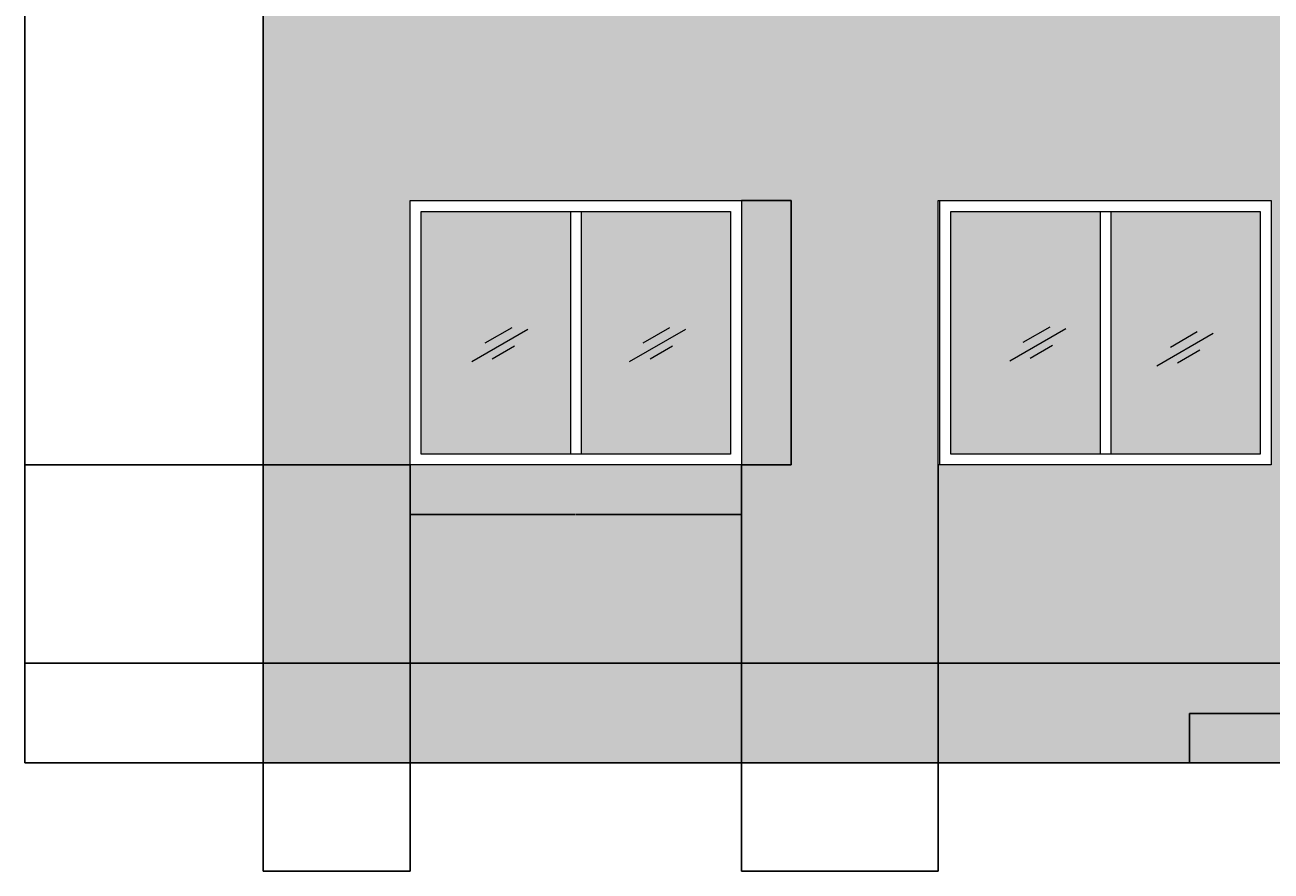
# Model space of a CAD drawing. Units: millimetres. Extents: x 2511 to 24632, y 2213 to 12972.
# Tile 4 of 5: x 13664 to 19414, y 2507 to 6412. Entities that reach past the tile are written whole.
import ezdxf

# ---------------------------------------------------------------- set-up
doc = ezdxf.new("R2010")
doc.units = ezdxf.units.MM
for name, color, linetype, lineweight in [('A-ANNO-DIMS', 2, 'Continuous', 18), ('A-BASE-PATT', 9, 'Continuous', 9), ('A-ELEV', 7, 'Continuous', 25), ('A-ELEV-GLAZ', 7, 'Continuous', 18), ('A-ELEV-PATT', 13, 'Continuous', 9)]:
    doc.layers.add(name, color=color, linetype=linetype, lineweight=lineweight)
doc.layers.add('A-GLAZ-PATT', color=141, linetype='Continuous', lineweight=9, true_color=0xadddf7)
doc.styles.get("Standard").update_dxf_attribs({"font": 'arial.ttf'})
doc.dimstyles.get("Standard").update_dxf_attribs({"dimtxt": 0.18, "dimasz": 0.18, "dimexe": 0.18, "dimexo": 0.0625, "dimgap": 0.09, "dimtad": 0, "dimtih": 1, "dimtoh": 1, "dimdec": 4, "dimzin": 0, "dimdsep": 46, "dimtxsty": 'Standard', "dimcen": 0.09, "dimadec": 0, "dimazin": 0, "dimtfac": 1, "dimtdec": 4, "dimtofl": 0, "dimtmove": 0, "dimatfit": 3, "dimfxl": 1, "dimtolj": 1, "dimtzin": 0, "dimarcsym": 0})

# ---------------------------------------------------------------- blocks, each defined once
blk = doc.blocks.new('WINDOW-FRAME-1528-ELEV')
for p, q in [((3.45580574503e-05, -0.0004698816292148), (3.45580574503e-05, 1219.999530118371)), ((3.45580574503e-05, 1219.999530118371), (1527.988197152912, 1219.999530118371)), ((1527.988197152912, 1219.999530118371), (1527.988197152912, -0.0004698816292148)), ((738.9941158554847, 1169.999530118371), (738.9941158554847, 49.99953011837078)), ((788.9941158554847, 1169.999530118371), (788.9941158554847, 49.99953011837078)), ((1527.988197152912, -0.0004698816292148), (3.45580574503e-05, -0.0004698816292148))]:
    blk.add_line(p, q)
for points in [[(3.45580574503e-05, 1219.999530118371), (1527.988197152912, 1219.999530118371), (1527.988197152912, -0.0004698816292148), (3.45580574503e-05, -0.0004698816292148)], [(50.00003455805745, 1169.999530118371), (1477.988197152912, 1169.999530118371), (1477.988197152912, 49.99953011837078), (50.00003455805745, 49.99953011837078)]]:
    blk.add_lwpolyline(points, close=True)
blk = doc.blocks.new('WINDOW-FRAME-1536-ELEV')
for p, q in [((-0.0001940248657775, -0.0004698816292148), (-0.0001940248657775, 1219.999530118371)), ((-0.0001940248657775, 1219.999530118371), (1536.172544795805, 1219.999530118371)), ((1536.172544795805, 1219.999530118371), (1536.172544795805, -0.0004698816292148)), ((747.1784634983741, 1169.999530118371), (747.1784634983741, 49.99953011837078)), ((797.1784634983742, 1169.999530118371), (797.1784634983742, 49.99953011837078)), ((1536.172544795805, -0.0004698816292148), (-0.0001940248657775, -0.0004698816292148))]:
    blk.add_line(p, q)
for points in [[(8.184382200950495, 1219.999530118371), (1536.172544795805, 1219.999530118371), (1536.172544795805, -0.0004698816292148), (8.184382200950495, -0.0004698816292148)], [(58.1843822009505, 1169.999530118371), (1486.172544795805, 1169.999530118371), (1486.172544795805, 49.99953011837078), (58.1843822009505, 49.99953011837078)]]:
    blk.add_lwpolyline(points, close=True)
blk = doc.blocks.new('GLASS-REFLECTION')
for p, q in [((0.000348498528183, -0.0002333358270334), (259.2110812861792, 149.655153015964)), ((62.47510116635385, 86.0291626371336), (186.2553756901197, 157.4937374537958)), ((94.69077173755068, 13.20916119840785), (197.7341820365163, 72.70130187273116))]:
    blk.add_line(p, q)
blk = doc.blocks.new('*D31')
at = {"layer": 'A-ANNO-DIMS', "color": 0, "lineweight": -2, "transparency": 16777216}
for p, q in [((15441.81503455806, 4381.154030118369), (15441.81503455806, 4151.838305729142)), ((16969.80319715291, 4381.154030118369), (16969.80319715291, 4151.838305729142)), ((15441.99503455805, 4152.018305729142), (16204.67128502329, 4152.018305729142)), ((16969.62319715291, 4152.018305729142), (16206.94694668768, 4152.018305729142))]:
    blk.add_line(p, q, dxfattribs=at)
at = {"layer": 'A-ANNO-DIMS', "color": 0, "transparency": 16777216}
for points in [[(15441.99503455805, 4152.048305729141), (15441.99503455805, 4151.988305729141), (15441.81503455806, 4152.018305729142)], [(16969.62319715291, 4152.048305729141), (16969.62319715291, 4151.988305729141), (16969.80319715291, 4152.018305729142)]]:
    blk.add_solid(points, dxfattribs=at)
at = {"layer": 'Defpoints', "color": 0, "transparency": 16777216}
for p in [(15441.81503455806, 4381.216530118369), (16969.80319715291, 4381.216530118369), (16969.80319715291, 4152.018305729142)]:
    blk.add_point(p, dxfattribs=at)
at = {"layer": 'A-ANNO-DIMS', "color": 0, "transparency": 16777216, "insert": (16205.80911585548, 4152.018305729142), "char_height": 0.18, "attachment_point": 5}
blk.add_mtext('\\A1;FRAME 1528 TYP.', dxfattribs=at)
blk = doc.blocks.new('*D32')
at = {"layer": 'A-ANNO-DIMS', "color": 0, "lineweight": -2, "transparency": 16777216}
for p, q in [((16969.86569715292, 5601.216530118371), (17199.18142154215, 5601.216530118371)), ((17199.00142154215, 5601.036530118371), (17199.00142154215, 4991.398433256161)), ((17199.00142154215, 4381.396530118371), (17199.00142154215, 4991.034626980582)), ((16969.86569715292, 4381.216530118371), (17199.18142154215, 4381.216530118371))]:
    blk.add_line(p, q, dxfattribs=at)
at = {"layer": 'A-ANNO-DIMS', "color": 0, "transparency": 16777216}
for points in [[(17198.97142154215, 5601.036530118371), (17199.03142154215, 5601.036530118371), (17199.00142154215, 5601.216530118371)], [(17198.97142154215, 4381.396530118371), (17199.03142154215, 4381.396530118371), (17199.00142154215, 4381.216530118371)]]:
    blk.add_solid(points, dxfattribs=at)
at = {"layer": 'Defpoints', "color": 0, "transparency": 16777216}
for p in [(16969.80319715292, 5601.216530118371), (17199.00142154215, 5601.216530118371), (16969.80319715292, 4381.216530118371)]:
    blk.add_point(p, dxfattribs=at)
at = {"layer": 'A-ANNO-DIMS', "color": 0, "transparency": 16777216, "insert": (17199.00142154215, 4991.216530118366), "char_height": 0.18, "attachment_point": 5}
blk.add_mtext('\\A1;1220 TYP.', dxfattribs=at)
blk = doc.blocks.new('*D66')
at = {"layer": 'A-ANNO-DIMS', "color": 0, "lineweight": -2, "transparency": 16777216}
for p, q in [((14762.747297, 3466.216530000002), (13663.87979700001, 3466.216530000002)), ((13664.05979700001, 3466.036530000002), (13664.05979700001, 3236.398433137792)), ((13664.05979700001, 3006.396530000001), (13664.05979700001, 3236.034626862212)), ((14762.747297, 3006.216530000001), (13663.87979700001, 3006.216530000001))]:
    blk.add_line(p, q, dxfattribs=at)
at = {"layer": 'A-ANNO-DIMS', "color": 0, "transparency": 16777216}
for points in [[(13664.02979700001, 3466.036530000002), (13664.08979700001, 3466.036530000002), (13664.05979700001, 3466.216530000002)], [(13664.02979700001, 3006.396530000001), (13664.08979700001, 3006.396530000001), (13664.05979700001, 3006.216530000001)]]:
    blk.add_solid(points, dxfattribs=at)
at = {"layer": 'Defpoints', "color": 0, "transparency": 16777216}
for p in [(13664.05979700001, 3466.216530000002), (14762.809797, 3466.216530000002), (14762.809797, 3006.216530000001)]:
    blk.add_point(p, dxfattribs=at)
at = {"layer": 'A-ANNO-DIMS', "color": 0, "transparency": 16777216, "insert": (13664.05979700001, 3236.216529999997), "char_height": 0.18, "attachment_point": 5}
blk.add_mtext('\\A1;460', dxfattribs=at)
blk = doc.blocks.new('*D67')
at = {"layer": 'A-ANNO-DIMS', "color": 0, "lineweight": -2, "transparency": 16777216}
for p, q in [((15441.75253500001, 4381.216530000002), (13663.87979700001, 4381.21653)), ((13664.05979700001, 4381.03653), (13664.05979700001, 3923.898433137792)), ((13664.05979700001, 3466.396530000003), (13664.05979700001, 3923.534626862211)), ((14762.747297, 3466.216530000002), (13663.87979700001, 3466.216530000002))]:
    blk.add_line(p, q, dxfattribs=at)
at = {"layer": 'A-ANNO-DIMS', "color": 0, "transparency": 16777216}
for points in [[(13664.02979700001, 4381.03653), (13664.08979700001, 4381.03653), (13664.05979700001, 4381.21653)], [(13664.02979700001, 3466.396530000003), (13664.08979700001, 3466.396530000003), (13664.05979700001, 3466.216530000002)]]:
    blk.add_solid(points, dxfattribs=at)
at = {"layer": 'Defpoints', "color": 0, "transparency": 16777216}
for p in [(13664.05979700001, 4381.21653), (15441.81503500001, 4381.216530000002), (14762.809797, 3466.216530000002)]:
    blk.add_point(p, dxfattribs=at)
at = {"layer": 'A-ANNO-DIMS', "color": 0, "transparency": 16777216, "insert": (13664.05979700001, 3923.716529999996), "char_height": 0.18, "attachment_point": 5}
blk.add_mtext('\\A1;915', dxfattribs=at)
blk = doc.blocks.new('*D68')
at = {"layer": 'A-ANNO-DIMS', "color": 0, "lineweight": -2, "transparency": 16777216}
for p, q in [((14762.747297, 6666.216530000004), (13663.87979700001, 6666.216530000003)), ((13664.05979700001, 6666.036530000003), (13664.05979700001, 5523.898433137791)), ((13664.05979700001, 4381.39653), (13664.05979700001, 5523.534626862211)), ((15441.75253500001, 4381.216530000002), (13663.87979700001, 4381.21653))]:
    blk.add_line(p, q, dxfattribs=at)
at = {"layer": 'A-ANNO-DIMS', "color": 0, "transparency": 16777216}
for points in [[(13664.02979700001, 6666.036530000003), (13664.08979700001, 6666.036530000003), (13664.05979700001, 6666.216530000003)], [(13664.02979700001, 4381.39653), (13664.08979700001, 4381.39653), (13664.05979700001, 4381.21653)]]:
    blk.add_solid(points, dxfattribs=at)
at = {"layer": 'Defpoints', "color": 0, "transparency": 16777216}
for p in [(13664.05979700001, 6666.216530000003), (14762.809797, 6666.216530000004), (15441.81503500001, 4381.216530000002)]:
    blk.add_point(p, dxfattribs=at)
at = {"layer": 'A-ANNO-DIMS', "color": 0, "transparency": 16777216, "insert": (13664.05979700001, 5523.716529999997), "char_height": 0.18, "attachment_point": 5}
blk.add_mtext('\\A1;2285', dxfattribs=at)
blk = doc.blocks.new('*D72')
at = {"layer": 'A-ANNO-DIMS', "color": 0, "lineweight": -2, "transparency": 16777216}
for p, q in [((15441.815035, 4381.15403), (15441.815035, 2507.28653)), ((14762.809797, 3006.15403), (14762.809797, 2507.28653)), ((14762.989797, 2507.46653), (15102.02289348977, 2507.46653)), ((15441.635035, 2507.46653), (15102.60193851023, 2507.46653))]:
    blk.add_line(p, q, dxfattribs=at)
at = {"layer": 'A-ANNO-DIMS', "color": 0, "transparency": 16777216}
for points in [[(14762.989797, 2507.49653), (14762.989797, 2507.43653), (14762.809797, 2507.46653)], [(15441.635035, 2507.49653), (15441.635035, 2507.43653), (15441.815035, 2507.46653)]]:
    blk.add_solid(points, dxfattribs=at)
at = {"layer": 'Defpoints', "color": 0, "transparency": 16777216}
for p in [(15441.815035, 4381.216529999999), (14762.809797, 3006.21653), (15441.815035, 2507.46653)]:
    blk.add_point(p, dxfattribs=at)
at = {"layer": 'A-ANNO-DIMS', "color": 0, "transparency": 16777216, "insert": (15102.312416, 2507.46653), "char_height": 0.18, "attachment_point": 5}
blk.add_mtext('\\A1;679', dxfattribs=at)
blk = doc.blocks.new('*D73')
at = {"layer": 'A-ANNO-DIMS', "color": 0, "lineweight": -2, "transparency": 16777216}
for p, q in [((16969.803197, 4381.15403), (16969.803197, 2507.28653)), ((17877.818806, 4381.15403), (17877.818806, 2507.28653)), ((16969.983197, 2507.46653), (17423.5219701221, 2507.46653)), ((17877.638806, 2507.46653), (17424.1000328779, 2507.46653))]:
    blk.add_line(p, q, dxfattribs=at)
at = {"layer": 'A-ANNO-DIMS', "color": 0, "transparency": 16777216}
for points in [[(16969.983197, 2507.49653), (16969.983197, 2507.43653), (16969.803197, 2507.46653)], [(17877.638806, 2507.49653), (17877.638806, 2507.43653), (17877.818806, 2507.46653)]]:
    blk.add_solid(points, dxfattribs=at)
at = {"layer": 'Defpoints', "color": 0, "transparency": 16777216}
for p in [(16969.803197, 4381.216529999999), (17877.818806, 4381.216529999999), (17877.818806, 2507.46653)]:
    blk.add_point(p, dxfattribs=at)
at = {"layer": 'A-ANNO-DIMS', "color": 0, "transparency": 16777216, "insert": (17423.8110015, 2507.46653), "char_height": 0.18, "attachment_point": 5}
blk.add_mtext('\\A1;908', dxfattribs=at)
blk = doc.blocks.new('*D80')
at = {"layer": 'A-ANNO-DIMS', "color": 0, "lineweight": -2, "transparency": 16777216}
for p, q in [((19536.424333, 3235.072051000002), (19037.55683300001, 3235.072051000002)), ((19037.73683300001, 3234.892051000001), (19037.73683300001, 3120.826193637791)), ((19037.73683300001, 3006.396530000001), (19037.73683300001, 3120.462387362211)), ((19536.424333, 3006.216530000001), (19037.55683300001, 3006.216530000001))]:
    blk.add_line(p, q, dxfattribs=at)
at = {"layer": 'A-ANNO-DIMS', "color": 0, "transparency": 16777216}
for points in [[(19037.70683300001, 3234.892051000001), (19037.76683300001, 3234.892051000001), (19037.73683300001, 3235.072051000002)], [(19037.70683300001, 3006.396530000001), (19037.76683300001, 3006.396530000001), (19037.73683300001, 3006.216530000001)]]:
    blk.add_solid(points, dxfattribs=at)
at = {"layer": 'Defpoints', "color": 0, "transparency": 16777216}
for p in [(19037.73683300001, 3235.072051000002), (19536.486833, 3235.072051000002), (19536.486833, 3006.216530000001)]:
    blk.add_point(p, dxfattribs=at)
at = {"layer": 'A-ANNO-DIMS', "color": 0, "transparency": 16777216, "insert": (19037.73683300001, 3120.644290499995), "char_height": 0.18, "attachment_point": 5}
blk.add_mtext('\\A1;228.86', dxfattribs=at)

msp = doc.modelspace()

# ---------------------------------------------------------------- hatches: boundary and pattern name
at = {"layer": 'A-BASE-PATT', "transparency": 33554595}
h = msp.add_hatch(color=256, dxfattribs=at)
h.dxf.hatch_style = 1
h.paths.add_polyline_path([(19536.48683262826, 3235.072050511866), (20721.84835936827, 3235.072050511866), (20721.84835936827, 3006.216530118372), (23532.80979657499, 3006.216530118372), (23938.80979657499, 3006.216530118372), (23938.80979657499, 3466.216530118371), (23532.80979657499, 3466.216530118371), (20718.80979657499, 3466.216530118371), (20718.80979657499, 3462.895537400881), (19843.80979657499, 3462.895537400881), (14762.80979657499, 3466.216530118371), (14762.80979657499, 3006.216530118372), (19536.48683262826, 3006.216530118372)])
at = {"layer": 'A-ELEV-PATT', "transparency": 33554551}
h = msp.add_hatch(color=256, dxfattribs=at)
h.dxf.hatch_style = 1
h.paths.add_polyline_path([(20858.80979657499, 6516.216530118374), (14762.80979657499, 6516.21653011837), (14762.80979657499, 3466.216530118371), (19843.80979657499, 3466.216530118371), (19843.80979657499, 5601.216530118371), (20718.80979657499, 5601.216530118371), (20718.80979657499, 3466.216530118371), (20858.80979657499, 3466.216530118371)])
h.paths.add_polyline_path([(16969.80319715291, 5601.216530118371), (16969.80319715291, 4381.21653011837), (15441.81503455806, 4381.21653011837), (15441.81503455806, 5601.216530118371)], flags=16)
h.paths.add_polyline_path([(16919.80319715291, 5551.21653011837), (16919.80319715291, 4431.21653011837), (15491.81503455806, 4431.21653011837), (15491.81503455806, 5551.21653011837)], flags=0)
h.paths.add_polyline_path([(17877.81880597513, 5601.216530118371), (19413.9915447958, 5601.216530118371), (19413.9915447958, 4381.21653011837), (17886.00338220095, 4381.21653011837), (17877.81880597513, 4381.21653011837)], flags=16)
h.paths.add_polyline_path([(17936.00338220095, 5551.21653011837), (19363.9915447958, 5551.21653011837), (19363.9915447958, 4431.21653011837), (17936.00338220095, 4431.21653011837)], flags=0)
h.paths.add_polyline_path([(20858.80979657499, 9716.216530118376), (14762.80979657499, 9716.21653011837), (14762.80979657499, 6666.21653011837), (19522.169078361, 6666.21653011837), (19522.169078361, 7733.216530118371), (20858.80979657499, 7733.216530118371)])
h.paths.add_polyline_path([(16969.80319715291, 8801.21653011837), (16969.80319715291, 7581.216530118371), (15441.81503455806, 7581.216530118371), (15441.81503455806, 8801.21653011837)], flags=16)
h.paths.add_polyline_path([(16919.80319715291, 8751.216530118369), (16919.80319715291, 7631.216530118371), (15491.81503455806, 7631.216530118371), (15491.81503455806, 8751.216530118369)], flags=0)
h.paths.add_polyline_path([(17877.81880597514, 8801.21653011837), (19413.9915447958, 8801.21653011837), (19413.9915447958, 7581.216530118371), (17886.00338220095, 7581.216530118371), (17877.81880597513, 7581.216530118371)], flags=16)
h.paths.add_polyline_path([(17936.00338220095, 8751.216530118369), (19363.9915447958, 8751.216530118369), (19363.9915447958, 7631.216530118371), (17936.00338220095, 7631.216530118371)], flags=0)
h.paths.add_polyline_path([(23051.60643531334, 9716.216530118376), (20858.80979657499, 9716.21653011837), (20858.80979657499, 7733.216530118371), (23051.60643531334, 7733.216530118371)])
h.paths.add_polyline_path([(23051.60643531335, 6516.216530118374), (20858.80979657499, 6516.216530118374), (20858.80979657499, 3516.21653011837), (23051.60643531335, 3516.21653011837)])
at = {"layer": 'A-GLAZ-PATT'}
h = msp.add_hatch(color=256, dxfattribs=at)
h.dxf.hatch_style = 1
h.paths.add_polyline_path([(16180.80911585549, 8751.216530118369), (15491.81503455806, 8751.216530118369), (15491.81503455806, 7631.216530118371), (16180.80911585549, 7631.216530118371)])
h.paths.add_polyline_path([(16919.80319715291, 8751.216530118369), (16230.80911585548, 8751.216530118369), (16230.80911585548, 7631.216530118371), (16919.80319715291, 7631.216530118371)])
h.paths.add_polyline_path([(18624.99746349838, 8751.216530118369), (17936.00338220095, 8751.216530118369), (17936.00338220095, 7631.216530118371), (18624.99746349838, 7631.216530118371)])
h.paths.add_polyline_path([(19363.9915447958, 8751.216530118369), (18674.99746349837, 8751.216530118369), (18674.99746349837, 7631.216530118371), (19363.9915447958, 7631.216530118371)])
h.paths.add_polyline_path([(16180.80911585548, 5551.21653011837), (15491.81503455806, 5551.21653011837), (15491.81503455806, 4431.21653011837), (16180.80911585548, 4431.21653011837)])
h.paths.add_polyline_path([(16919.80319715291, 5551.21653011837), (16230.80911585548, 5551.21653011837), (16230.80911585548, 4431.21653011837), (16919.80319715291, 4431.21653011837)])
h.paths.add_polyline_path([(18624.99746349837, 5551.21653011837), (17936.00338220095, 5551.21653011837), (17936.00338220095, 4431.21653011837), (18624.99746349837, 4431.21653011837)])
h.paths.add_polyline_path([(19363.9915447958, 5551.21653011837), (18674.99746349837, 5551.21653011837), (18674.99746349837, 4431.21653011837), (19363.9915447958, 4431.21653011837)])

# ---------------------------------------------------------------- linework, layer by layer
at = {"layer": 'A-ELEV'}
for p, q in [((14762.80979657499, 3466.216530118371), (14762.80979657499, 7733.216530118371)), ((14762.80979657499, 3466.216530118371), (23532.80979657499, 3466.216530118371)), ((14762.80979657499, 3006.216530118369), (14762.80979657499, 3466.216530118371)), ((14762.80979657499, 3006.216530118372), (23532.80979657499, 3006.216530118372))]:
    msp.add_line(p, q, dxfattribs=at)

# ---------------------------------------------------------------- block references
at = {"layer": 'A-ELEV-GLAZ'}
for name, p in [('WINDOW-FRAME-1528-ELEV', (15441.815, 4381.216999999999)), ('WINDOW-FRAME-1536-ELEV', (17877.819, 4381.216999999999)), ('GLASS-REFLECTION', (15725.32052761088, 4857.903827074651)), ('GLASS-REFLECTION', (16453.73598216432, 4857.903827074651)), ('GLASS-REFLECTION', (18207.97937281527, 4861.092869066835)), ('GLASS-REFLECTION', (18887.35323147503, 4839.204974318707))]:
    msp.add_blockref(name, p, dxfattribs=at)

# ---------------------------------------------------------------- dimensions: what is measured, and where the dimension line sits
at = {"layer": 'A-ANNO-DIMS'}
for base, p1, p2, override, picture, middle in [((13664.05979700001, 6666.216530000003), (15441.815035, 4381.216529999999), (14762.809797, 6666.216529999999), {"dimdec": 0, "dimlfac": 1, "dimrnd": 0, "dimzin": 0, "dimdsep": 46, "dimlunit": 2}, '*D68', (13664.05979700001, 5523.716529999997)), ((13664.05979700001, 4381.21653), (14762.809797, 3466.21653), (15441.815035, 4381.216529999999), {"dimdec": 0, "dimlfac": 1, "dimrnd": 0, "dimzin": 0, "dimdsep": 46, "dimlunit": 2}, '*D67', (13664.05979700001, 3923.716529999996)), ((13664.05979700001, 3466.216530000002), (14762.809797, 3006.21653), (14762.809797, 3466.21653), {"dimdec": 0, "dimlfac": 1, "dimrnd": 0, "dimzin": 0, "dimdsep": 46, "dimlunit": 2}, '*D66', (13664.05979700001, 3236.216529999997)), ((19037.73683300001, 3235.072051000002), (19536.486833, 3006.21653), (19536.486833, 3235.072051), {"dimdec": 2, "dimlfac": 1, "dimrnd": 0, "dimzin": 0, "dimdsep": 46, "dimlunit": 2}, '*D80', (19037.73683300001, 3120.644290499995))]:
    dim = msp.add_linear_dim(base=base, p1=p1, p2=p2, angle=90, dimstyle='Standard', override=override, dxfattribs=at)
    dim.commit()
    dim.dimension.update_dxf_attribs({"geometry": picture, "text_midpoint": middle})
dim = msp.add_linear_dim(base=(17199.00142154215, 5601.216530118371), p1=(16969.80319715291, 4381.216530118369), p2=(16969.80319715291, 5601.21653011837), angle=90, text='<> TYP.', dimstyle='Standard', override={"dimdec": 0, "dimlfac": 1, "dimrnd": 0, "dimzin": 0, "dimdsep": 46, "dimlunit": 2}, dxfattribs=at)
dim.commit()
dim.dimension.update_dxf_attribs({"geometry": '*D32', "text_midpoint": (17199.00142154215, 4991.216530118366)})
for base, p1, p2, picture, middle in [((15441.815035, 2507.46653), (14762.809797, 3006.21653), (15441.815035, 4381.216529999999), '*D72', (15102.312416, 2507.46653)), ((17877.818806, 2507.46653), (16969.803197, 4381.216529999999), (17877.818806, 4381.216529999999), '*D73', (17423.8110015, 2507.46653))]:
    dim = msp.add_linear_dim(base=base, p1=p1, p2=p2, dimstyle='Standard', override={"dimdec": 0, "dimlfac": 1, "dimrnd": 0, "dimzin": 0, "dimdsep": 46, "dimlunit": 2}, dxfattribs=at)
    dim.commit()
    dim.dimension.update_dxf_attribs({"geometry": picture, "text_midpoint": middle})
dim = msp.add_linear_dim(base=(16969.80319715291, 4152.018305729142), p1=(15441.81503455806, 4381.216530118369), p2=(16969.80319715291, 4381.216530118369), text='FRAME <> TYP.', dimstyle='Standard', override={"dimdec": 0, "dimlfac": 1, "dimrnd": 0, "dimzin": 0, "dimdsep": 46, "dimlunit": 2}, dxfattribs=at)
dim.commit()
dim.dimension.update_dxf_attribs({"geometry": '*D31', "text_midpoint": (16205.80911585548, 4152.018305729142)})

doc.saveas('drawing.dxf')
